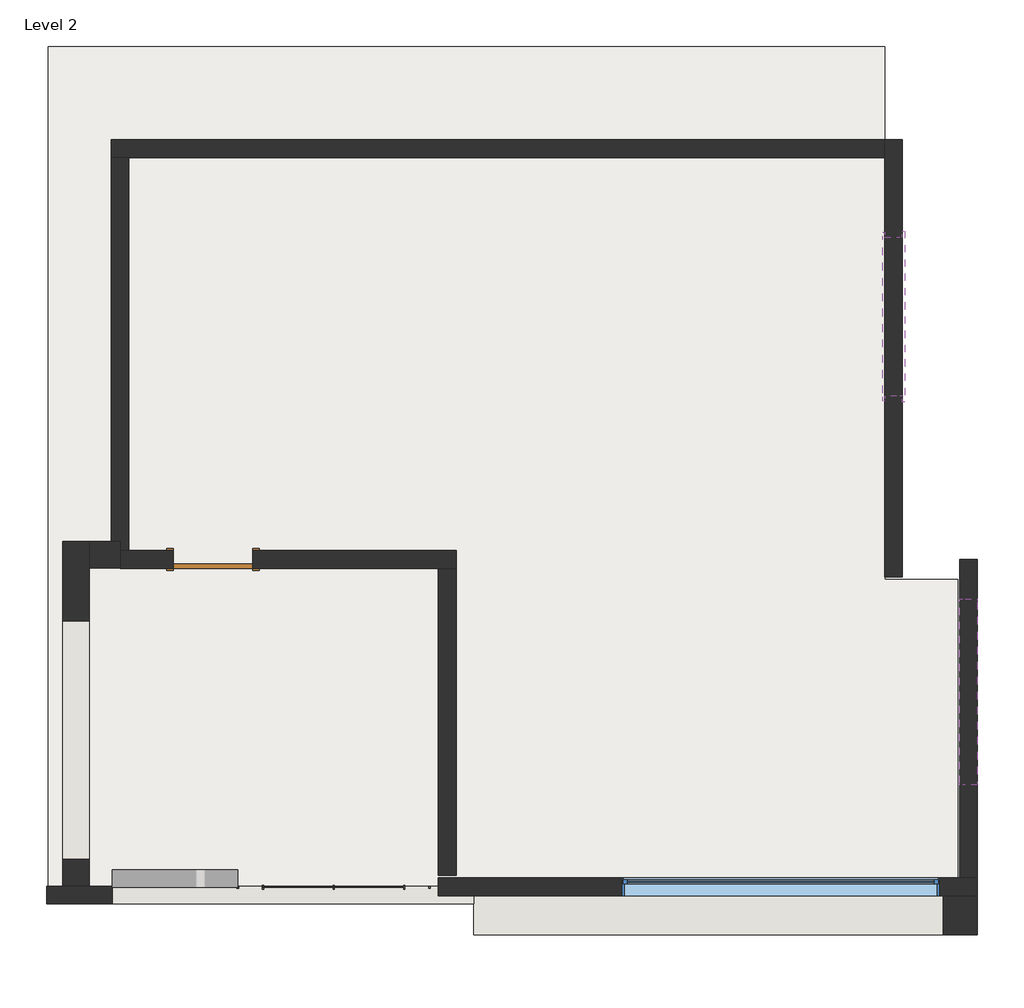
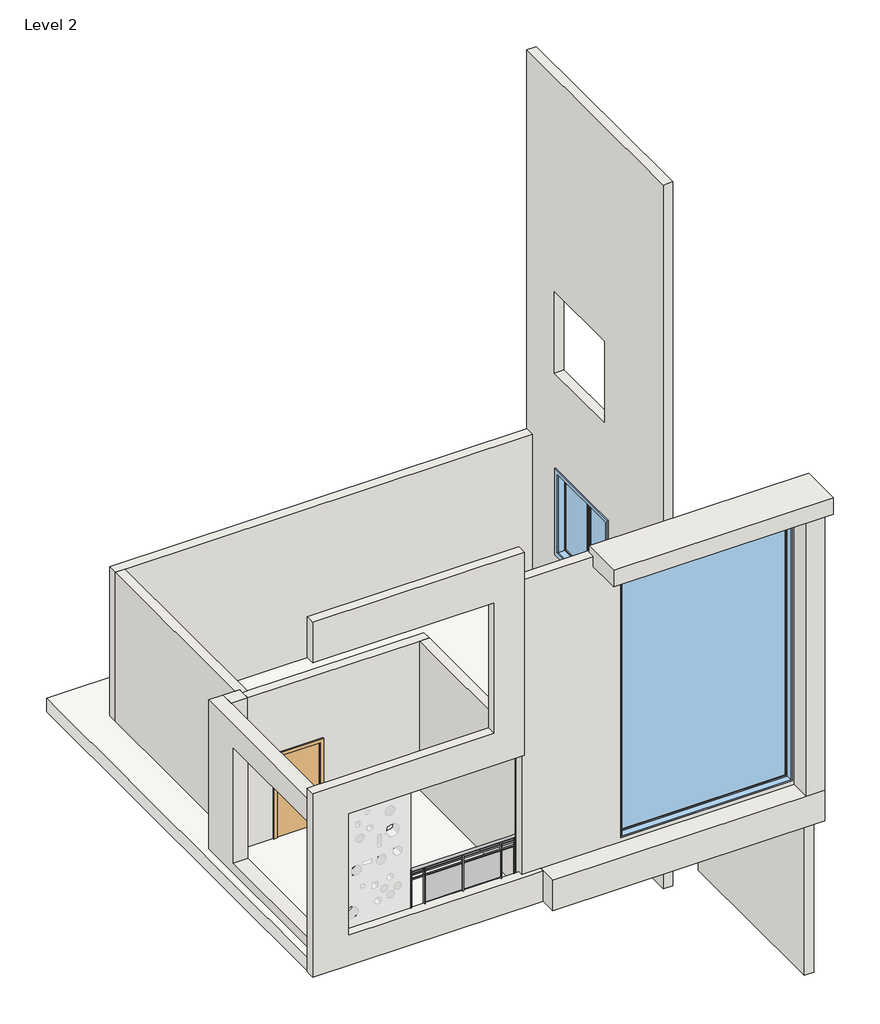
# One storey, part 2 of 2: 11 walls, 3 windows, 1 door, 1 railing, 1 roof.
"""IFC4 building model written with IfcOpenShell, lengths in millimetres."""

from ifc_helpers import new_model, si_unit, point, frame, origin, place, context, project, spatial, polyline, ellipse_curve, trimmed, outline, extrude, faceted_brep, transform, mapped, element, save
from ifc_brep_helpers import plane_surface, extruded_surface, advanced_brep
from components import door_54dd4da4, walls_1_walls_1_d5e167dd, window_b085ff8d, window_c349b51b, window_a973ac2f

model = new_model("IFC4")

# Units and contexts
model_context = context("Model", 3, world=origin())
ifc_project = project(units=[si_unit("LENGTHUNIT", "METRE", prefix="MILLI")], contexts=[model_context])

# Site, building, storey
site = spatial("IfcSite", under=ifc_project)
building = spatial("IfcBuilding", under=site)
storey = spatial("IfcBuildingStorey", under=building, Name="Level 2", Elevation=3657.6)

# Door
placement = place(None, origin())
door_shape = door_54dd4da4(model_context)
element("IfcDoor", 1, ObjectType="Single-Flush : 36\" x 84\"", at=placement, inside=storey, context=model_context, shape_type="MappedRepresentation", body=[
    mapped(door_shape, transform((-8945.7821198, 5315.00098, 3657.6), x_axis=(-1.0, 0.0, 0.0), y_axis=(0.0, -1.0, 0.0), z_axis=(0.0, 0.0, 1.0))),
])

# Railing
element("IfcRailing", 2, ObjectType="Glass Panel - Bottom Fill", at=placement, inside=storey, context=model_context, shape_type="SolidModel", body=[
    advanced_brep(
    [(-8663.1307892, 1582.3572776, 5181.6), (-8663.1307892, 1506.1572776, 5181.6), (-6453.3307892, 1582.3572776, 5181.6), (-6453.3307892, 1506.1572776, 5181.6)],
    [
        (0, 1, ellipse_curve(frame((-8663.1307892, 1544.2572776, 5181.6), z_axis=(-1.0, 0.0, 0.0), x_axis=(0.0, -1.0, 0.0)), 38.1, 28.575)),
        (1, 0, ellipse_curve(frame((-8663.1307892, 1544.2572776, 5181.6), z_axis=(-1.0, 0.0, 0.0), x_axis=(0.0, -1.0, 0.0)), 38.1, 28.575)),
        (2, 3, ellipse_curve(frame((-6453.3307892, 1544.2572776, 5181.6), z_axis=(1.0, 0.0, 0.0), x_axis=(0.0, -1.0, 0.0)), 38.1, 28.575)),
        (3, 2, ellipse_curve(frame((-6453.3307892, 1544.2572776, 5181.6), z_axis=(1.0, 0.0, 0.0), x_axis=(0.0, -1.0, 0.0)), 38.1, 28.575)),
        (0, 2),
        (3, 1),
    ],
    [
        plane_surface(frame((-8663.1307892, 1544.2572776, 5181.6), z_axis=(-1.0, 0.0, 0.0), x_axis=(0.0, 1.0, 0.0))),
        plane_surface(frame((-6453.3307892, 1544.2572776, 5181.6), z_axis=(1.0, 0.0, 0.0), x_axis=(0.0, 1.0, 0.0))),
        extruded_surface(trimmed(ellipse_curve(frame((-6453.3307892, 1544.2572776, 5181.6), z_axis=(-1.0, 0.0, 0.0), x_axis=(0.0, -1.0, 0.0)), 38.1, 28.575), [point((-6453.3307892, 1582.3572776, 5181.6))], [point((-6453.3307892, 1506.1572776, 5181.6))], True, "CARTESIAN"), (-2209.8, 0.0, 0.0), 2209.8),
        extruded_surface(trimmed(ellipse_curve(frame((-6453.3307892, 1544.2572776, 5181.6), z_axis=(-1.0, 0.0, 0.0), x_axis=(0.0, -1.0, 0.0)), 38.1, 28.575), [point((-6453.3307892, 1506.1572776, 5181.6))], [point((-6453.3307892, 1582.3572776, 5181.6))], True, "CARTESIAN"), (-2209.8, 0.0, 0.0), 2209.8),
    ],
    [
        (0, [[1, 2]]),
        (1, [[3, 4]]),
        (2, [[-1, 5, -4, 6]]),
        (3, [[-2, -6, -3, -5]]),
    ],
),
    extrude(outline(polyline([(-8663.1307892, 1531.5572776), (-8663.1307892, 1556.9572776), (-6453.3307892, 1556.9572776), (-6453.3307892, 1531.5572776), (-8663.1307892, 1531.5572776)])), frame((0.0, 0.0, 5067.3), z_axis=(0.0, 0.0, 1.0), x_axis=(1.0, 0.0, 0.0)), (0.0, 0.0, 1.0), 25.4),
    extrude(outline(polyline([(-8663.1307892, 1531.5572776), (-8663.1307892, 1556.9572776), (-6453.3307892, 1556.9572776), (-6453.3307892, 1531.5572776), (-8663.1307892, 1531.5572776)])), frame((0.0, 0.0, 4965.7), z_axis=(0.0, 0.0, 1.0), x_axis=(1.0, 0.0, 0.0)), (0.0, 0.0, 1.0), 25.4),
    extrude(outline(polyline([(-6751.7807892, 1518.8572776), (-6751.7807892, 1569.6572776), (-6739.0807892, 1569.6572776), (-6739.0807892, 1518.8572776), (-6751.7807892, 1518.8572776)])), frame((0.0, 0.0, 4267.2), z_axis=(0.0, 0.0, 1.0), x_axis=(1.0, 0.0, 0.0)), (0.0, 0.0, 1.0), 885.6788223),
    extrude(outline(polyline([(-7558.2307892, 1550.7924346), (-6745.4307892, 1550.7924346), (-6745.4307892, 1544.4424346), (-7558.2307892, 1544.4424346), (-7558.2307892, 1550.7924346)])), frame((0.0, 0.0, 4368.8), z_axis=(0.0, 0.0, 1.0), x_axis=(1.0, 0.0, 0.0)), (0.0, 0.0, 1.0), 596.9),
    extrude(outline(polyline([(-7564.5807892, 1518.8572776), (-7564.5807892, 1569.6572776), (-7551.8807892, 1569.6572776), (-7551.8807892, 1518.8572776), (-7564.5807892, 1518.8572776)])), frame((0.0, 0.0, 4267.2), z_axis=(0.0, 0.0, 1.0), x_axis=(1.0, 0.0, 0.0)), (0.0, 0.0, 1.0), 885.6788223),
    extrude(outline(polyline([(-8371.0307892, 1550.7924346), (-7558.2307892, 1550.7924346), (-7558.2307892, 1544.4424346), (-8371.0307892, 1544.4424346), (-8371.0307892, 1550.7924346)])), frame((0.0, 0.0, 4368.8), z_axis=(0.0, 0.0, 1.0), x_axis=(1.0, 0.0, 0.0)), (0.0, 0.0, 1.0), 596.9),
    extrude(outline(polyline([(-8377.3807892, 1518.8572776), (-8377.3807892, 1569.6572776), (-8364.6807892, 1569.6572776), (-8364.6807892, 1518.8572776), (-8377.3807892, 1518.8572776)])), frame((0.0, 0.0, 4267.2), z_axis=(0.0, 0.0, 1.0), x_axis=(1.0, 0.0, 0.0)), (0.0, 0.0, 1.0), 885.6788223),
    extrude(outline(polyline([(-6466.0307892, 1534.7322776), (-6466.0307892, 1553.7822776), (-6446.9807892, 1553.7822776), (-6446.9807892, 1534.7322776), (-6466.0307892, 1534.7322776)])), frame((0.0, 0.0, 4267.2), z_axis=(0.0, 0.0, 1.0), x_axis=(1.0, 0.0, 0.0)), (0.0, 0.0, 1.0), 885.6788223),
    extrude(outline(polyline([(-8669.4807892, 1534.7322776), (-8669.4807892, 1553.7822776), (-8650.4307892, 1553.7822776), (-8650.4307892, 1534.7322776), (-8669.4807892, 1534.7322776)])), frame((0.0, 0.0, 4267.2), z_axis=(0.0, 0.0, 1.0), x_axis=(1.0, 0.0, 0.0)), (0.0, 0.0, 1.0), 885.6788223),
])

# Roof
element("IfcRoof", 3, ObjectType="Generic - 12\"", at=placement, inside=storey, context=model_context, shape_type="SweptSolid", body=[
    extrude(outline(polyline([(-10836.7012689, 11214.3911137), (-1224.1821198, 11214.3911137), (-1224.1821198, 5086.40098), (-385.9821198, 5086.40098), (-385.9821198, 1387.3881635), (-10836.7012689, 1387.3881635), (-10836.7012689, 11214.3911137)])), frame((0.0, 0.0, 3657.6), z_axis=(0.0, 0.0, 1.0), x_axis=(1.0, 0.0, 0.0)), (0.0, 0.0, 1.0), 304.8),
])

# Walls
element("IfcWall", 4, ObjectType="Generic - 12\"", at=placement, inside=storey, context=model_context, shape_type="Brep", body=[
    faceted_brep([(-10368.1932957, 1558.4652184, 3657.6), (-10368.1932957, 5216.0652184, 3657.6), (-10368.1932957, 5520.8652184, 3657.6), (-10368.1932957, 5520.8652184, 7315.2), (-10368.1932957, 5216.0652184, 7315.2), (-10368.1932957, 1558.4652184, 7315.2), (-10368.1932957, 1866.5256437, 6782.8581243), (-10368.1932957, 4609.7256437, 6782.8581243), (-10368.1932957, 4609.7256437, 4192.0581243), (-10368.1932957, 1866.5256437, 4192.0581243), (-10672.9932957, 1558.4652184, 3657.6), (-10672.9932957, 1558.4652184, 7315.2), (-10672.9932957, 5520.8652184, 7315.2), (-10672.9932957, 5520.8652184, 3657.6), (-10672.9932957, 1866.5256437, 6782.8581243), (-10672.9932957, 1866.5256437, 4192.0581243), (-10672.9932957, 4609.7256437, 4192.0581243), (-10672.9932957, 4609.7256437, 6782.8581243)], [[[0, 1, 2, 3, 4, 5], [6, 7, 8, 9]], [[10, 11, 12, 13], [14, 15, 16, 17]], [[0, 5, 11, 10]], [[2, 1, 0, 10, 13]], [[5, 4, 3, 12, 11]], [[7, 6, 14, 17]], [[8, 7, 17, 16]], [[9, 8, 16, 15]], [[6, 9, 15, 14]], [[3, 2, 13, 12]]]),
])
element("IfcWall", 5, ObjectType="Generic - 12\"", at=placement, inside=storey, context=model_context, shape_type="Brep", body=[
    faceted_brep([(-10368.1932957, 5216.0652184, 3657.6), (-10012.5821198, 5216.0652184, 3657.6), (-10012.5821198, 5216.0652184, 7315.2), (-10368.1932957, 5216.0652184, 7315.2), (-10368.1932957, 5520.8652184, 3657.6), (-10368.1932957, 5520.8652184, 7315.2), (-10114.1821198, 5520.8652184, 7315.2), (-10012.5821198, 5520.8652184, 7315.2), (-10012.5821198, 5520.8652184, 3657.6), (-10114.1821198, 5520.8652184, 3657.6), (-10012.5821198, 5416.60098, 3657.6), (-10012.5821198, 5416.60098, 7315.2)], [[[0, 1, 2, 3]], [[4, 5, 6, 7, 8, 9]], [[1, 0, 4, 9, 8, 10]], [[2, 1, 10, 8, 7, 11]], [[3, 2, 11, 7, 6, 5]], [[0, 3, 5, 4]]]),
])
element("IfcWall", 6, ObjectType="Generic - 8\"", at=placement, inside=storey, context=model_context, shape_type="Brep", body=[
    faceted_brep([(-10114.1821198, 9937.80098, 3657.6), (-9910.9821198, 9937.80098, 3657.6), (-1224.1821198, 9937.80098, 3657.6), (-1224.1821198, 9937.80098, 7315.2), (-9910.9821198, 9937.80098, 7315.2), (-10114.1821198, 9937.80098, 7315.2), (-10114.1821198, 10141.00098, 3657.6), (-10114.1821198, 10141.00098, 7315.2), (-1224.1821198, 10141.00098, 7315.2), (-1224.1821198, 10141.00098, 3657.6)], [[[0, 1, 2, 3, 4, 5]], [[6, 7, 8, 9]], [[2, 1, 0, 6, 9]], [[5, 4, 3, 8, 7]], [[0, 5, 7, 6]], [[3, 2, 9, 8]]]),
])
element("IfcWall", 7, ObjectType="Generic - 8\"", at=placement, inside=storey, context=model_context, shape_type="SweptSolid", body=[
    extrude(outline(polyline([(-9910.9821198, 9937.80098), (-9910.9821198, 5416.60098), (-10012.5821198, 5416.60098), (-10012.5821198, 5520.8652184), (-10114.1821198, 5520.8652184), (-10114.1821198, 9937.80098), (-9910.9821198, 9937.80098)])), frame((0.0, 0.0, 3657.6), z_axis=(0.0, 0.0, 1.0), x_axis=(1.0, 0.0, 0.0)), (0.0, 0.0, 1.0), 3657.6),
])
element("IfcWall", 8, ObjectType="Generic - 8\"", at=placement, inside=storey, context=model_context, shape_type="Brep", body=[
    faceted_brep([(-157.3821198, 1650.6780349, 3657.6), (-360.5821198, 1650.6780349, 3657.6), (-6354.9821198, 1650.6780349, 3657.6), (-6354.9821198, 1650.6780349, 7315.2), (-6354.9821198, 1650.6780349, 10972.8), (-6253.3821198, 1650.6780349, 10972.8), (-360.5821198, 1650.6780349, 10972.8), (-157.3821198, 1650.6780349, 10972.8), (-157.3821198, 1650.6780349, 7315.2), (-589.1821198, 1650.6780349, 4435.5856227), (-589.1821198, 1650.6780349, 10531.5856227), (-4246.7821198, 1650.6780349, 10531.5856227), (-4246.7821198, 1650.6780349, 4435.5856227), (-6354.9821198, 1447.4780349, 3657.6), (-157.3821198, 1447.4780349, 3657.6), (-157.3821198, 1447.4780349, 10972.8), (-6354.9821198, 1447.4780349, 10972.8), (-589.1821198, 1447.4780349, 10531.5856227), (-589.1821198, 1447.4780349, 4435.5856227), (-4246.7821198, 1447.4780349, 4435.5856227), (-4246.7821198, 1447.4780349, 10531.5856227), (-6354.9821198, 1558.4652184, 10972.8), (-157.3821198, 1558.4652184, 10972.8)], [[[0, 1, 2, 3, 4, 5, 6, 7, 8], [9, 10, 11, 12]], [[13, 14, 15, 16], [17, 18, 19, 20]], [[2, 1, 0, 14, 13]], [[7, 6, 5, 4, 21, 16, 15, 22]], [[2, 13, 16, 21, 4, 3]], [[17, 10, 9, 18]], [[18, 9, 12, 19]], [[19, 12, 11, 20]], [[10, 17, 20, 11]], [[14, 0, 8, 7, 22, 15]]]),
])
element("IfcWall", 9, ObjectType="Generic - 8\"", at=placement, inside=storey, context=model_context, shape_type="Brep", body=[
    faceted_brep([(-360.5821198, 5315.00098, 0.0), (-360.5821198, 5111.80098, 0.0), (-360.5821198, 1606.60098, 0.0), (-360.5821198, 1403.40098, 0.0), (-360.5821198, 1403.40098, 3657.6), (-360.5821198, 1606.60098, 3657.6), (-360.5821198, 1650.6780349, 3657.6), (-360.5821198, 1650.6780349, 7315.2), (-360.5821198, 2724.20098, 7315.2), (-360.5821198, 2724.20098, 6256.6655485), (-360.5821198, 4857.80098, 6256.6655485), (-360.5821198, 4857.80098, 7315.2), (-360.5821198, 5111.80098, 7315.2), (-360.5821198, 5315.00098, 7315.2), (-360.5821198, 4857.80098, 3624.7438024), (-360.5821198, 2724.20098, 3624.7438024), (-360.5821198, 2724.20098, 2405.5438024), (-360.5821198, 4857.80098, 2405.5438024), (-157.3821198, 1403.40098, 0.0), (-157.3821198, 5315.00098, 0.0), (-157.3821198, 5315.00098, 7315.2), (-157.3821198, 5111.80098, 7315.2), (-157.3821198, 4857.80098, 7315.2), (-157.3821198, 4857.80098, 6256.6655485), (-157.3821198, 2724.20098, 6256.6655485), (-157.3821198, 2724.20098, 7315.2), (-157.3821198, 1650.6780349, 7315.2), (-157.3821198, 1650.6780349, 3657.6), (-157.3821198, 1447.4780349, 3657.6), (-157.3821198, 1403.40098, 3657.6), (-157.3821198, 4857.80098, 3624.7438024), (-157.3821198, 4857.80098, 2405.5438024), (-157.3821198, 2724.20098, 2405.5438024), (-157.3821198, 2724.20098, 3624.7438024)], [[[0, 1, 2, 3, 4, 5, 6, 7, 8, 9, 10, 11, 12, 13], [14, 15, 16, 17]], [[18, 19, 20, 21, 22, 23, 24, 25, 26, 27, 28, 29], [30, 31, 32, 33]], [[3, 2, 1, 0, 19, 18]], [[7, 26, 25, 8]], [[20, 13, 12, 11, 22, 21]], [[0, 13, 20, 19]], [[3, 18, 29, 4]], [[26, 7, 6, 27]], [[6, 5, 4, 29, 28, 27]], [[31, 30, 14, 17]], [[32, 31, 17, 16]], [[33, 32, 16, 15]], [[30, 33, 15, 14]], [[10, 23, 22, 11]], [[23, 10, 9, 24]], [[24, 9, 8, 25]]]),
])
element("IfcWall", 10, ObjectType="Generic - 8\"", at=placement, inside=storey, context=model_context, shape_type="Brep", body=[
    faceted_brep([(-10012.5821198, 5213.40098, 3657.6), (-9402.9821198, 5213.40098, 3657.6), (-9402.9821198, 5213.40098, 5791.2), (-8488.5821198, 5213.40098, 5791.2), (-8488.5821198, 5213.40098, 3657.6), (-6354.9821198, 5213.40098, 3657.6), (-6151.7821198, 5213.40098, 3657.6), (-6151.7821198, 5213.40098, 7315.2), (-6354.9821198, 5213.40098, 7315.2), (-10012.5821198, 5213.40098, 7315.2), (-9402.9821198, 5416.60098, 5791.2), (-9402.9821198, 5416.60098, 3657.6), (-9910.9821198, 5416.60098, 3657.6), (-10012.5821198, 5416.60098, 3657.6), (-10012.5821198, 5416.60098, 7315.2), (-9910.9821198, 5416.60098, 7315.2), (-6151.7821198, 5416.60098, 7315.2), (-6151.7821198, 5416.60098, 3657.6), (-8488.5821198, 5416.60098, 3657.6), (-8488.5821198, 5416.60098, 5791.2), (-10012.5821198, 5216.0652184, 3657.6), (-10012.5821198, 5216.0652184, 7315.2)], [[[0, 1, 2, 3, 4, 5, 6, 7, 8, 9]], [[10, 11, 12, 13, 14, 15, 16, 17, 18, 19]], [[18, 17, 6, 5, 4]], [[13, 12, 11, 1, 0, 20]], [[9, 8, 7, 16, 15, 14, 21]], [[0, 9, 21, 14, 13, 20]], [[7, 6, 17, 16]], [[2, 1, 11, 10]], [[3, 2, 10, 19]], [[4, 3, 19, 18]]]),
])
element("IfcWall", 11, ObjectType="Generic - 8\"", at=placement, inside=storey, context=model_context, shape_type="SweptSolid", body=[
    extrude(outline(polyline([(-6354.9821198, 1682.80098), (-6354.9821198, 5213.40098), (-6151.7821198, 5213.40098), (-6151.7821198, 1682.80098), (-6354.9821198, 1682.80098)])), frame((0.0, 0.0, 3657.6), z_axis=(0.0, 0.0, 1.0), x_axis=(1.0, 0.0, 0.0)), (0.0, 0.0, 1.0), 3657.6),
])
element("IfcWall", 12, ObjectType="Generic - 8\"", at=placement, inside=storey, context=model_context, shape_type="Brep", body=[
    faceted_brep([(-10858.7268197, 1355.2652184, 10744.2), (-6989.9932957, 1355.2652184, 10744.2), (-6989.9932957, 1355.2652184, 7797.8), (-10858.7268197, 1355.2652184, 7797.8), (-10858.7268197, 1355.2652184, 3657.6), (-5949.9629707, 1355.2652184, 3657.6), (-5949.9629707, 1355.2652184, 4341.7312703), (-6354.9821198, 1355.2652184, 4341.7312703), (-10102.8741466, 1355.2652184, 4341.7312703), (-10102.8741466, 1355.2652184, 7084.9312703), (-6354.9821198, 1355.2652184, 7084.9312703), (-6354.9821198, 1355.2652184, 11656.9312703), (-10858.7268197, 1355.2652184, 11656.9312703), (-10858.7268197, 1558.4652184, 10744.2), (-10858.7268197, 1558.4652184, 11656.9312703), (-6354.9821198, 1558.4652184, 11656.9312703), (-6354.9821198, 1558.4652184, 10972.8), (-6354.9821198, 1558.4652184, 7315.2), (-6354.9821198, 1558.4652184, 7084.9312703), (-10102.8741466, 1558.4652184, 7084.9312703), (-10102.8741466, 1558.4652184, 4341.7312703), (-6354.9821198, 1558.4652184, 4341.7312703), (-5949.9629707, 1558.4652184, 4341.7312703), (-5949.9629707, 1558.4652184, 3657.6), (-10368.1932957, 1558.4652184, 3657.6), (-10672.9932957, 1558.4652184, 3657.6), (-10858.7268197, 1558.4652184, 3657.6), (-10858.7268197, 1558.4652184, 7797.8), (-10672.9932957, 1558.4652184, 7797.8), (-10368.1932957, 1558.4652184, 7797.8), (-6989.9932957, 1558.4652184, 7797.8), (-6989.9932957, 1558.4652184, 10744.2), (-10368.1932957, 1558.4652184, 10744.2), (-10672.9932957, 1558.4652184, 10744.2), (-10102.8741466, 1544.2572776, 4341.7312703), (-10102.8741466, 1544.2572776, 7084.9312703)], [[[0, 1, 2, 3, 4, 5, 6, 7, 8, 9, 10, 11, 12]], [[13, 14, 15, 16, 17, 18, 19, 20, 21, 22, 23, 24, 25, 26, 27, 28, 29, 30, 31, 32, 33]], [[5, 4, 26, 25, 24, 23]], [[12, 11, 15, 14]], [[0, 12, 14, 13]], [[1, 0, 13, 33, 32, 31]], [[2, 1, 31, 30]], [[3, 2, 30, 29, 28, 27]], [[4, 3, 27, 26]], [[6, 5, 23, 22]], [[8, 7, 6, 22, 21, 20, 34]], [[10, 9, 35, 19, 18]], [[10, 18, 17, 16, 15, 11]], [[8, 34, 20, 19, 35, 9]]]),
])
element("IfcWall", 13, ObjectType="Generic - 8\"", at=placement, inside=storey, context=model_context, shape_type="Brep", body=[
    faceted_brep([(-1224.1821198, 10141.00098, 15849.6), (-1224.1821198, 10141.00098, 14630.4), (-1224.1821198, 10141.00098, 11150.0899101), (-1224.1821198, 10141.00098, 10972.8), (-1224.1821198, 10141.00098, 7315.2), (-1224.1821198, 10141.00098, 3657.6), (-1224.1821198, 10141.00098, 0.0), (-1224.1821198, 9937.80098, 0.0), (-1224.1821198, 5111.80098, 0.0), (-1224.1821198, 5111.80098, 14630.4), (-1224.1821198, 5111.80098, 15849.6), (-1224.1821198, 5315.00098, 15849.6), (-1224.1821198, 9937.80098, 15849.6), (-1224.1821198, 7296.20098, 11012.3075998), (-1224.1821198, 7296.20098, 9183.5075998), (-1224.1821198, 9125.00098, 9183.5075998), (-1224.1821198, 9125.00098, 11012.3075998), (-1224.1821198, 7194.60098, 7017.2039084), (-1224.1821198, 7194.60098, 5188.4039084), (-1224.1821198, 9023.40098, 5188.4039084), (-1224.1821198, 9023.40098, 7017.2039084), (-1224.1821198, 7220.00098, 3048.0), (-1224.1821198, 7220.00098, 1219.2), (-1224.1821198, 9048.80098, 1219.2), (-1224.1821198, 9048.80098, 3048.0), (-1020.9821198, 10141.00098, 0.0), (-1020.9821198, 10141.00098, 15849.6), (-1020.9821198, 5315.00098, 15849.6), (-1020.9821198, 5111.80098, 15849.6), (-1020.9821198, 5111.80098, 0.0), (-1020.9821198, 5315.00098, 0.0), (-1020.9821198, 7296.20098, 11012.3075998), (-1020.9821198, 9125.00098, 11012.3075998), (-1020.9821198, 9125.00098, 9183.5075998), (-1020.9821198, 7296.20098, 9183.5075998), (-1020.9821198, 7194.60098, 7017.2039084), (-1020.9821198, 9023.40098, 7017.2039084), (-1020.9821198, 9023.40098, 5188.4039084), (-1020.9821198, 7194.60098, 5188.4039084), (-1020.9821198, 7220.00098, 3048.0), (-1020.9821198, 9048.80098, 3048.0), (-1020.9821198, 9048.80098, 1219.2), (-1020.9821198, 7220.00098, 1219.2)], [[[0, 1, 2, 3, 4, 5, 6, 7, 8, 9, 10, 11, 12], [13, 14, 15, 16], [17, 18, 19, 20], [21, 22, 23, 24]], [[25, 26, 27, 28, 29, 30], [31, 32, 33, 34], [35, 36, 37, 38], [39, 40, 41, 42]], [[8, 7, 6, 25, 30, 29]], [[0, 12, 11, 10, 28, 27, 26]], [[8, 29, 28, 10, 9]], [[0, 26, 25, 6, 5, 4, 3, 2, 1]], [[14, 13, 31, 34]], [[15, 14, 34, 33]], [[16, 15, 33, 32]], [[13, 16, 32, 31]], [[18, 17, 35, 38]], [[19, 18, 38, 37]], [[20, 19, 37, 36]], [[17, 20, 36, 35]], [[22, 21, 39, 42]], [[23, 22, 42, 41]], [[24, 23, 41, 40]], [[21, 24, 40, 39]]]),
])
walls_1_walls_1_shape = walls_1_walls_1_d5e167dd(model_context)
element("IfcWall", 14, ObjectType="Walls 1 : Walls 1", at=placement, inside=storey, context=model_context, shape_type="MappedRepresentation", body=[
    mapped(walls_1_walls_1_shape, transform((0.0, 152.4, 0.0), x_axis=(1.0, 0.0, 0.0), y_axis=(0.0, 1.0, 0.0), z_axis=(0.0, 0.0, 1.0))),
])

# Windows
window_shape = window_b085ff8d(model_context)
element("IfcWindow", 15, ObjectType="Casement Dbl with Trim : 72\" x 36\"", at=placement, inside=storey, context=model_context, shape_type="MappedRepresentation", body=[
    mapped(window_shape, transform((-1141.6321198, 8109.00098, 3969.2039084), x_axis=(0.0, -1.0, 0.0), y_axis=(1.0, 0.0, 0.0), z_axis=(0.0, 0.0, 1.0))),
])
window_2_shape = window_c349b51b(model_context)
element("IfcWindow", 16, ObjectType="Fixed : 36\" x 48\"", at=placement, inside=storey, context=model_context, shape_type="MappedRepresentation", body=[
    mapped(window_2_shape, transform((-2379.8821198, 1549.0780349, 3521.1856227), x_axis=(1.0, 0.0, 0.0), y_axis=(0.0, 1.0, 0.0), z_axis=(0.0, 0.0, 1.0))),
])
window_3_shape = window_a973ac2f(model_context)
element("IfcWindow", 17, ObjectType="Fixed : 36\" x 72\"", at=placement, inside=storey, context=model_context, shape_type="MappedRepresentation", body=[
    mapped(window_3_shape, transform((-258.9821198, 3829.10098, 5951.8655485), x_axis=(0.0, 1.0, 0.0), y_axis=(-1.0, 0.0, 0.0), z_axis=(0.0, 0.0, 1.0))),
])

save(model, "model.ifc")

# Revit data of these elements
# Type "Single-Flush : 36\" x 84\""
#   Type Mark = "1"
#   Construction Type Id = "MDOOR"
#   Assembly Code = "C1020"
#   Analytic Construction = "Metal"
#   Thickness = 0' - 2"
#   Heat Transfer Coefficient (U) = 0.651978 BTU/(h·ft²·°F)
#   Height = 7' - 0"
#   Trim Projection Ext = 0' - 1"
#   Trim Projection Int = 0' - 1"
#   Trim Width = 0' - 3"
#   Width = 3' - 0"
#   Define Thermal Properties by = 1
#   Door Material = Door - Panel
#   Frame Material = Door - Frame
#   Visual Light Transmittance = 0
#   Solar Heat Gain Coefficient = 0
#   Function = (empty or 0)
#   Wall Closure = (empty or 0)
# Type "Glass Panel - Bottom Fill"
#   Assembly Code = "C2010400"
#   built-in parameter 1008612 = 0.0416667 (stored number, unit not read)
#   built-in parameter 1008611 = 0.0416667 (stored number, unit not read)
#   built-in parameter 1008609 = 0.333333 (stored number, unit not read)
#   built-in parameter 1008604 = 0.166667 (stored number, unit not read)
#   built-in parameter 1008603 = 0.166667 (stored number, unit not read)
#   Railing Height = 3' - 0"
#   built-in parameter 1008630 = 2
#   built-in parameter 1008610 = 2
#   built-in parameter 1008618 = Baluster - Square : 3/4"
# Type "Generic - 12\""
#   Assembly Code = "B1020"
#   Layers, outside or top first: 1' - 0" no material (function 1)
# Type "Generic - 12\""
#   Assembly Code = "B2010"
#   Layers, outside or top first: 1' - 0" no material (function 1)
# Type "Generic - 8\""
#   Assembly Code = "B2010"
#   Layers, outside or top first: 0' - 8" no material (function 1)
# Type "Casement Dbl with Trim : 72\" x 36\""
#   Type Mark = "11"
#   Construction Type Id = "GSP4R"
#   Assembly Code = "B2020100"
#   Analytic Construction = "1/8 in Pilkington single glazing"
#   Visual Light Transmittance = 0.9
#   Solar Heat Gain Coefficient = 0.78
#   Heat Transfer Coefficient (U) = 0.6496 BTU/(h·ft²·°F)
#   Height = 6' - 0"
#   Default Sill Height = 4' - 0"
#   Trim Projection - Ext. = 0' - 0 1/2"
#   Trim Projection - Int. = 0' - 0 3/4"
#   Trim Width - Exterior = 0' - 3 1/2"
#   Trim Width - Interior = 0' - 3 1/2"
#   Width = 6' - 0"
#   Window Inset = 0' - 0 3/4"
#   Define Thermal Properties by = 1
#   Glass Pane Material = Glass
#   Sash Material = Sash
#   Trim Exterior Material = Trim
#   Trim Interior Material = Trim
#   Wall Closure = (empty or 0)
# Type "Fixed : 36\" x 48\""
#   Type Mark = "1"
#   Construction Type Id = "GSP4R"
#   Assembly Code = "B2020100"
#   Analytic Construction = "1/8 in Pilkington single glazing"
#   Visual Light Transmittance = 0.9
#   Solar Heat Gain Coefficient = 0.78
#   Heat Transfer Coefficient (U) = 0.6496 BTU/(h·ft²·°F)
#   Height = 20' - 0"
#   Default Sill Height = 3' - 0"
#   Width = 12' - 0"
#   Window Inset = 0' - 0 3/4"
#   Define Thermal Properties by = 1
#   Glass Pane Material = Glass
#   Sash Material = Sash
#   Wall Closure = (empty or 0)
# Type "Fixed : 36\" x 72\""
#   Type Mark = "9"
#   Construction Type Id = "GSP4R"
#   Assembly Code = "B2020100"
#   Analytic Construction = "1/8 in Pilkington single glazing"
#   Visual Light Transmittance = 0.9
#   Solar Heat Gain Coefficient = 0.78
#   Heat Transfer Coefficient (U) = 0.6496 BTU/(h·ft²·°F)
#   Height = 4' - 0"
#   Default Sill Height = 1' - 0"
#   Width = 7' - 0"
#   Window Inset = 0' - 0 3/4"
#   Define Thermal Properties by = 1
#   Glass Pane Material = Glass
#   Sash Material = Sash
#   Wall Closure = (empty or 0)
# Element 1 (IfcDoor, "Single-Flush : 36\" x 84\"")
#   Phase Created = New Construction
#   Materials on its faces: "Door - Frame", "Door - Panel"
# Element 2 (IfcRailing, "Glass Panel - Bottom Fill")
#   built-in parameter 1008621 = 2 (stored number, unit not read)
#   Phase Created = New Construction
#   Materials on its faces: "Glass"
# Element 3 (IfcRoof, "Generic - 12\"")
#   built-in parameter 1001705 = 13 (stored number, unit not read)
#   built-in parameter 1001710 = 33615
#   Phase Created = New Construction
#   Materials on its faces: "Default Roof"
# Elements 4, 5 (IfcWall, "Generic - 12\"")
#   Top Offset = 0' - 0"
#   Base Offset = 0' - 0"
#   Unconnected Height = 12' - 0"
#   wall height = 12' - 0"
#   Phase Created = New Construction
#   Base Constraint = Level 2
#   Materials on its faces: "Default Wall"
# Elements 6, 7, 10, 11 (IfcWall, "Generic - 8\"")
#   Top Offset = 0' - 0"
#   Base Offset = 0' - 0"
#   Unconnected Height = 12' - 0"
#   wall height = 12' - 0"
#   Phase Created = New Construction
#   Base Constraint = Level 2
#   Materials on its faces: "Default Wall"
# Element 8 (IfcWall, "Generic - 8\"")
#   Top Offset = 0' - 0"
#   Base Offset = 0' - 0"
#   Unconnected Height = 24' - 0"
#   wall height = 24' - 0"
#   Phase Created = New Construction
#   Base Constraint = Level 2
#   Materials on its faces: "Default Wall", "Laminate, Ivory, Matte"
# Element 9 (IfcWall, "Generic - 8\"")
#   built-in parameter 1001111 = -12' - 0"
#   Top Offset = 0' - 0"
#   Base Offset = -12' - 0"
#   Unconnected Height = 24' - 0"
#   wall height = 24' - 0"
#   Phase Created = New Construction
#   Base Constraint = Level 2
#   Materials on its faces: "Default Wall", "Laminate, Ivory, Matte"
# Element 12 (IfcWall, "Generic - 8\"")
#   Top Offset = 0' - 0"
#   Base Offset = 0' - 0"
#   Unconnected Height = 26' - 2.9343"
#   wall height = 26' - 2.9343"
#   Phase Created = New Construction
#   Base Constraint = Level 2
#   Materials on its faces: "Default Wall", "Laminate, Ivory, Matte"
# Element 13 (IfcWall, "Generic - 8\"")
#   built-in parameter 1001111 = -12' - 0"
#   Top Offset = 0' - 0"
#   Base Offset = -12' - 0"
#   Unconnected Height = 52' - 0"
#   wall height = 52' - 0"
#   Phase Created = New Construction
#   Base Constraint = Level 2
#   Materials on its faces: "Default Wall", "Earth"
# Element 14 (IfcWall, "Walls 1 : Walls 1")
#   Phase Created = New Construction
#   Materials on its faces: "Default Wall"
# Element 15 (IfcWindow, "Casement Dbl with Trim : 72\" x 36\"")
#   Mark = "9"
#   Phase Created = New Construction
#   Materials on its faces: "Sash", "Trim", "Glass"
# Element 16 (IfcWindow, "Fixed : 36\" x 48\"")
#   Mark = "2"
#   Phase Created = New Construction
#   Materials on its faces: "Sash", "Glass"
# Element 17 (IfcWindow, "Fixed : 36\" x 72\"")
#   Mark = "4"
#   Phase Created = New Construction
#   Materials on its faces: "Sash", "Glass"
# Materials
#   "Door - Panel": class "Wood", colour RGB 210 159 95, transparency 0
#   "Door - Frame": colour RGB 118 70 51, transparency 0
#   "Glass": class "Glass", colour RGB 0 128 192, transparency 0.75, Description = "Soda Lime Glass", Cost = 0
#   "Sash": class "Wood", colour RGB 224 178 126, transparency 0
#   "Trim": class "Wood", colour RGB 224 178 126, transparency 0
#   "Default Roof": colour RGB 88 101 114, transparency 0
#   "Default Wall": colour RGB 128 128 128, transparency 0
#   "Laminate, Ivory, Matte": class "Plastic", colour RGB 247 247 239, transparency 0, Description = "Plastic Laminate - Ivory, Matte", Cost = 0
#   "Earth": class "Generic", colour RGB 97 75 62, transparency 0, Description = "Soil", Cost = 0
